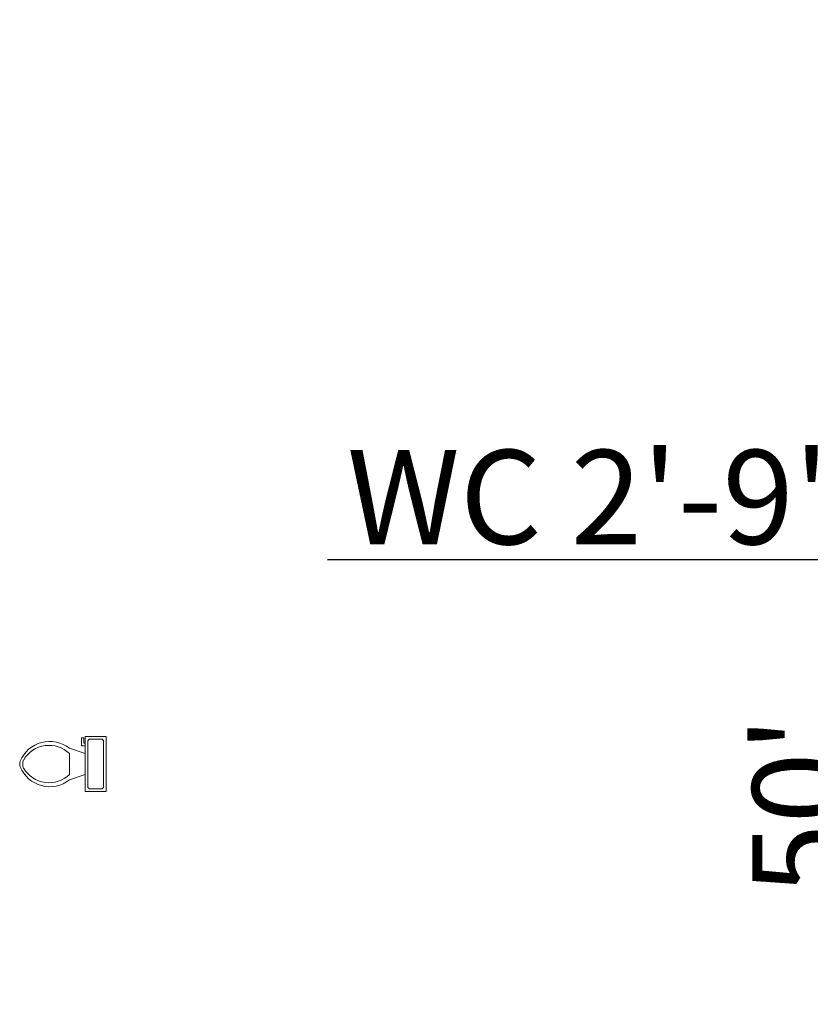
# Model space of a CAD drawing. Units: inches. Extents: x 2901 to 21549, y 2042 to 3828.
# Tile 2 of 10: x 2901 to 3202, y 3099 to 3474. Entities that reach past the tile are written whole.
import ezdxf

# ---------------------------------------------------------------- set-up
doc = ezdxf.new("R2010")
doc.units = ezdxf.units.IN
doc.layers.get('Defpoints').update_dxf_attribs({"color": 1})
doc.layers.add('A-ANNO-DIMS', color=2, linetype='Continuous', lineweight=18)
doc.layers.add('A-FLOR-FIXT', color=9, linetype='Continuous', lineweight=18)
doc.styles.get("Standard").update_dxf_attribs({"font": 'arial.ttf'})
doc.dimstyles.new('ISO-25', dxfattribs={"dimtxt": 36, "dimasz": 5, "dimexe": 1.25, "dimexo": 0.625, "dimtad": 1, "dimdec": 0, "dimlunit": 3, "dimtxsty": 'Standard', "dimcen": 2.5, "dimadec": 0, "dimazin": 0, "dimtfac": 1, "dimtdec": 0, "dimtmove": 0, "dimatfit": 3, "dimfxl": 1, "dimarcsym": 0})

# ---------------------------------------------------------------- blocks, each defined once
blk = doc.blocks.new('Toilet - top')
for p, q in [((9.5, -6), (9.5, -2)), ((-10, -8.5), (-8, -8.5)), ((-10, -9.5), (-10, -8.5)), ((-7, -9.5), (-10, -9.5)), ((-8, -8.5), (-8, -8)), ((-7, -8), (-7, -9.5)), ((-4, -8), (-6, -14)), ((4, -8), (6, -14)), ((4, -14), (-4, -14))]:
    blk.add_line(p, q)
blk.add_lwpolyline([(10.5, -8), (10.5, 0), (-10.5, 0), (-10.5, -8)], close=True)
for points in [[(-9.5, -2), (-9.5, -6)], [(8.5, -1), (-8.5, -1)], [(-8.5, -7), (8.5, -7)]]:
    blk.add_lwpolyline(points)
for centre, radius, start, end in [((-8.62, -1.88), 0.884, 81.8699, 188.1301), ((8.62, -1.88), 0.884, 351.8699, 98.1301), ((-8.62, -6.12), 0.884, 171.8699, 278.1301), ((8.62, -6.12), 0.884, 261.8699, 8.1301), ((3.52, -21.58), 12.17, 141.4691, 247.9714), ((4.2, -21.82), 11.33, 136.3677, 238.9468), ((-3.52, -21.58), 12.17, 292.0284, 38.5307), ((-4.2, -21.82), 11.33, 301.053, 43.6321), ((0, -27.88), 4, 245.7318, 294.2682), ((0, -29), 4, 254.8605, 285.1395)]:
    blk.add_arc(centre, radius, start, end)
blk = doc.blocks.new('*D31')
at = {"layer": 'A-ANNO-DIMS', "color": 0, "lineweight": -2, "transparency": 16777216}
for p, q in [((3333.44, 3474.48), (3220.78, 3474.48)), ((3222.03, 3469.48), (3222.03, 2879.48)), ((3333.44, 2874.48), (3220.78, 2874.48))]:
    blk.add_line(p, q, dxfattribs=at)
at = {"layer": 'A-ANNO-DIMS', "color": 0, "transparency": 16777216}
for points in [[(3221.19, 3469.48), (3222.86, 3469.48), (3222.03, 3474.48)], [(3221.19, 2879.48), (3222.86, 2879.48), (3222.03, 2874.48)]]:
    blk.add_solid(points, dxfattribs=at)
at = {"layer": 'Defpoints', "color": 0, "transparency": 16777216}
for p in [(3334.07, 3474.48), (3222.03, 2874.48), (3334.07, 2874.48)]:
    blk.add_point(p, dxfattribs=at)
at = {"layer": 'A-ANNO-DIMS', "color": 0, "transparency": 16777216, "insert": (3203.02, 3174.48), "char_height": 36, "attachment_point": 5, "rotation": 90}
blk.add_mtext("50'", dxfattribs=at)
blk = doc.blocks.new('*D40')
at = {"layer": 'A-ANNO-DIMS', "color": 0, "lineweight": -2, "transparency": 16777216}
for p, q in [((3343.07, 3272.69), (3343.07, 3267.11)), ((3376.12, 3272.69), (3376.12, 3267.11)), ((3343.07, 3268.36), (3018.15, 3268.36)), ((3371.12, 3268.36), (3348.07, 3268.36))]:
    blk.add_line(p, q, dxfattribs=at)
at = {"layer": 'A-ANNO-DIMS', "color": 0, "transparency": 16777216}
for points in [[(3348.07, 3269.19), (3348.07, 3267.52), (3343.07, 3268.36)], [(3371.12, 3269.19), (3371.12, 3267.52), (3376.12, 3268.36)]]:
    blk.add_solid(points, dxfattribs=at)
at = {"layer": 'Defpoints', "color": 0, "transparency": 16777216}
for p in [(3343.07, 3273.32), (3376.12, 3273.32), (3343.07, 3268.36)]:
    blk.add_point(p, dxfattribs=at)
at = {"layer": 'A-ANNO-DIMS', "color": 0, "transparency": 16777216, "insert": (3178.11, 3287.6), "char_height": 36, "attachment_point": 5}
blk.add_mtext('WC 2\'-9" TYP.', dxfattribs=at)

msp = doc.modelspace()

# ---------------------------------------------------------------- block references
at = {"layer": 'A-FLOR-FIXT', "rotation": 270}
msp.add_blockref('Toilet - top', (2933.58, 3190.4), dxfattribs=at)

# ---------------------------------------------------------------- dimensions: what is measured, and where the dimension line sits
at = {"layer": 'A-ANNO-DIMS'}
dim = msp.add_linear_dim(base=(3222.03, 2874.48), p1=(3334.07, 3474.48), p2=(3334.07, 2874.48), angle=90, dimstyle='ISO-25', override={"dimclrd": 0, "dimclre": 0, "dimclrt": 0}, dxfattribs=at)
dim.commit()
dim.dimension.update_dxf_attribs({"geometry": '*D31', "text_midpoint": (3203.02, 3174.48)})
dim = msp.add_linear_dim(base=(3343.0696, 3268.3583), p1=(3376.1159, 3273.3152), p2=(3343.0696, 3273.3152), angle=180, text='WC <> TYP.', dimstyle='ISO-25', override={"dimdec": 1, "dimlfac": 1, "dimrnd": 0, "dimzin": 1, "dimdsep": 46, "dimlunit": 4, "dimfrac": 2}, dxfattribs=at)
dim.commit()
dim.dimension.update_dxf_attribs({"geometry": '*D40', "text_midpoint": (3178.109, 3287.5972)})

doc.saveas('drawing.dxf')
